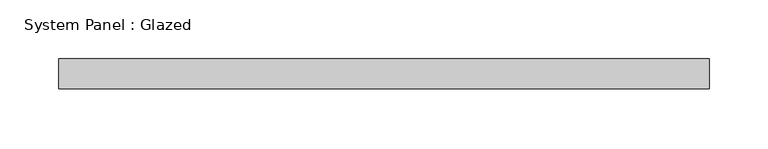
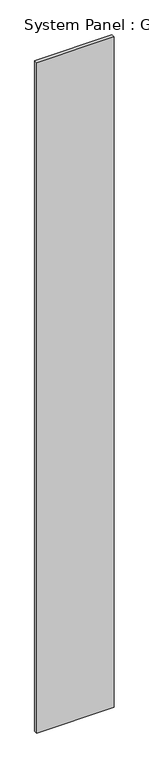
"""IFC4 building model written with IfcOpenShell, lengths in millimetres: plate geometry, System Panel : Glazed."""

from ifc_helpers import new_model, si_unit, origin, origin_with_axes, place, context, project, spatial, polyline, outline, extrude, source, transform, mapped, element, save


def system_panel_glazed_ecbfc98a(model_context):
    return source(origin(), model_context, "Body", "SweptSolid", [
        extrude(outline(polyline([(275.9422868, 19.05), (-275.9422868, 19.05), (-275.9422868, 44.45), (275.9422868, 44.45), (275.9422868, 19.05)])), origin_with_axes(), (0.0, 0.0, 1.0), 5054.6),
    ])


if __name__ == "__main__":
    model = new_model("IFC4")
    model_context = context("Model", 3, world=origin())
    ifc_project = project(units=[si_unit("LENGTHUNIT", "METRE", prefix="MILLI")], contexts=[model_context])
    site = spatial("IfcSite", under=ifc_project)
    building = spatial("IfcBuilding", under=site)
    placement = place(None, origin())
    system_panel_glazed_shape = system_panel_glazed_ecbfc98a(model_context)
    element("IfcPlate", 1, ObjectType="System Panel : Glazed", at=placement, inside=building, context=model_context, shape_type="MappedRepresentation", body=[
        mapped(system_panel_glazed_shape, transform((0.0, 0.0, 0.0), x_axis=(1.0, 0.0, 0.0), y_axis=(0.0, 1.0, 0.0), z_axis=(0.0, 0.0, 1.0))),
    ])
    save(model, "model.ifc")

# Revit data of these elements
# Type "System Panel : Glazed"
#   Construction Type Id = "GSP4R"
#   Analytic Construction = "1/8 in Pilkington single glazing"
#   Visual Light Transmittance = 0.9
#   Solar Heat Gain Coefficient = 0.86
#   Heat Transfer Coefficient (U) = 1.18115 BTU/(h·ft²·°F)
# Element 1 (IfcPlate, "System Panel : Glazed")
#   Materials on its faces: "Glass"
# Materials
#   "Glass": class "Glass", colour RGB 0 128 192, transparency 0.75, Description = "Soda Lime Glass", Cost = 0
